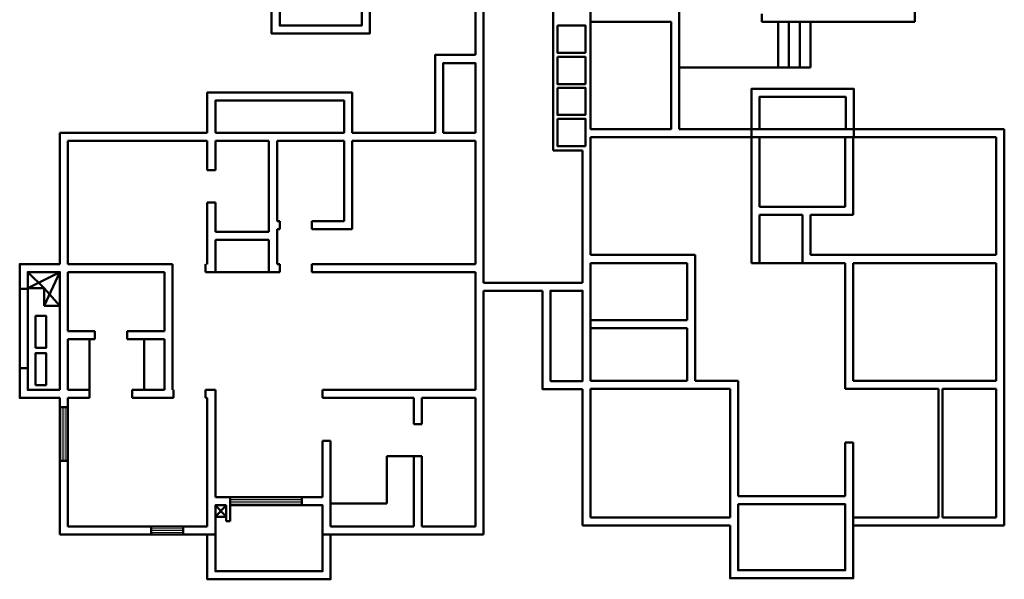
# Model space of a CAD drawing. Units: inches. Extents: x -105 to 1531, y -656 to 2003.
# Tile 1 of 6: x -105 to 997, y -656 to -29. Entities that reach past the tile are written whole.
import ezdxf

# ---------------------------------------------------------------- set-up
doc = ezdxf.new("R2010")
doc.units = ezdxf.units.IN
doc.header["$MEASUREMENT"] = 0
doc.layers.add('A-GLAZ', color=4, linetype='Continuous', lineweight=18)
doc.layers.add('A-WALL', color=7, linetype='Continuous', lineweight=50)

msp = doc.modelspace()

# ---------------------------------------------------------------- linework, layer by layer
at = {"layer": 'A-GLAZ'}
for p, q in [((105, -303), (102.8, -303)), ((105, -303), (102.8, -303)), ((102.8, -312), (105, -312)), ((-57.5, -523.3), (-57.5, -463.3)), ((-55.5, -523.3), (-55.5, -463.3)), ((-53.5, -523.3), (-53.5, -463.3)), ((-51, -463.3), (-51, -523.3)), ((130.5, -566.5), (210.6, -566.5)), ((130.5, -568.5), (210.6, -568.5)), ((130.5, -570.5), (210.6, -570.5)), ((42.1, -599.5), (78.1, -599.5)), ((42.1, -601.5), (78.1, -601.5)), ((42.1, -603.5), (78.1, -603.5))]:
    msp.add_line(p, q, dxfattribs=at)
at = {"layer": 'A-WALL'}
for p, q in [((897, -31.9), (897, 112.1)), ((492, -31.9), (492, 67.1)), ((534, -31.9), (534, 49.1)), ((633, -31.9), (633, 35.6)), ((277.8, -36), (277.8, 0)), ((405, -69), (405, 0)), ((414, 0), (414, -78)), ((492, -31.9), (492, -175.9)), ((534, -31.9), (534, -151.9)), ((624, -31.9), (534, -31.9)), ((633, -31.9), (633, -151.9)), ((725.8, -22.9), (725.8, -31.9)), ((897, -31.9), (725.8, -31.9)), ((744, -82.9), (744, -31.9)), ((756, -82.9), (756, -31.9)), ((768, -82.9), (768, -31.9)), ((780, -82.9), (780, -31.9)), ((405, -78), (369, -78)), ((369, -78), (369, -156)), ((405, -156), (405, -78)), ((414, -78), (414, -156)), ((780, -82.9), (633, -82.9)), ((258, -156), (258, -120)), ((723, -151.9), (723, -115.9)), ((534, -151.9), (624, -151.9)), ((633, -151.9), (997, -151.9)), ((997, -151.9), (997, -595.9)), ((-60, -156), (-60, -303)), ((105, -156), (-60, -156)), ((-51, -165), (-51, -303)), ((105, -165), (-51, -165)), ((105, -165), (105, -198)), ((258, -156), (114, -156)), ((114, -165), (114, -198)), ((174, -165), (114, -165)), ((174, -165), (174, -267)), ((183, -165), (183, -255)), ((258, -165), (183, -165)), ((258, -165), (258, -255)), ((360, -156), (267, -156)), ((405, -165), (267, -165)), ((267, -165), (267, -264)), ((405, -156), (369, -156)), ((405, -165), (405, -303)), ((414, -156), (414, -323.9)), ((534, -160.9), (534, -175.9)), ((633, -160.9), (534, -160.9)), ((534, -160.9), (714, -160.9)), ((534, -160.9), (534, -292.9)), ((714, -160.9), (714, -301.9)), ((723, -160.9), (723, -238.9)), ((723, -160.9), (819, -160.9)), ((819, -160.9), (819, -238.9)), ((828, -160.9), (828, -247.9)), ((828, -160.9), (988, -160.9)), ((988, -160.9), (988, -292.9)), ((492, -175.9), (525, -175.9)), ((525, -175.9), (525, -323.9)), ((534, -175.9), (534, -292.9)), ((114, -198), (105, -198)), ((105, -234), (114, -234)), ((105, -234), (105, -303)), ((114, -234), (114, -267)), ((723, -238.9), (819, -238.9)), ((723, -247.9), (771, -247.9)), ((723, -247.9), (723, -301.9)), ((771, -247.9), (771, -301.9)), ((780, -247.9), (780, -292.9)), ((780, -247.9), (828, -247.9)), ((186, -255), (183, -255)), ((183, -264), (183, -303)), ((186, -264), (183, -264)), ((186, -255), (186, -264)), ((258, -255), (222, -255)), ((222, -264), (222, -255)), ((267, -264), (222, -264)), ((174, -267), (114, -267)), ((174, -276), (114, -276)), ((114, -276), (114, -312)), ((174, -276), (174, -312)), ((534, -292.9), (651, -292.9)), ((651, -292.9), (651, -433.9)), ((780, -292.9), (988, -292.9)), ((66, -303), (-51, -303)), ((66, -312), (66, -303)), ((102.8, -303), (102.8, -312)), ((186, -303), (183, -303)), ((186, -303), (186, -312)), ((405, -303), (222, -303)), ((222, -312), (222, -303)), ((534, -301.9), (642, -301.9)), ((534, -301.9), (534, -365.9)), ((534, -301.9), (534, -332.9)), ((642, -301.9), (642, -365.9)), ((714, -301.9), (819, -301.9)), ((819, -301.9), (819, -442.9)), ((828, -301.9), (828, -433.9)), ((828, -301.9), (988, -301.9)), ((988, -301.9), (988, -433.9)), ((-60, -312), (-96, -312)), ((-96, -312), (-96, -330)), ((-60, -312), (-96, -330)), ((-96, -330), (-96, -312)), ((-96, -312), (-77.7, -330)), ((-77.7, -350), (-60, -312)), ((-60, -312), (-60, -444)), ((57, -312), (-51, -312)), ((-51, -312), (-51, -378)), ((57, -312), (57, -378)), ((66, -312), (66, -444)), ((186, -312), (102.8, -312)), ((405, -312), (222, -312)), ((405, -312), (405, -444)), ((-96, -330), (-77.7, -330)), ((-77.7, -330), (-77.7, -350)), ((-77.7, -330), (-60, -350)), ((525, -323.9), (414, -323.9)), ((-105, -330.8), (-96, -330.8)), ((-96, -330.8), (-96, -419.5)), ((480, -332.9), (414, -332.9)), ((414, -332.9), (414, -606)), ((525, -332.9), (489, -332.9)), ((525, -332.9), (525, -434.1)), ((534, -332.9), (534, -365.9)), ((-77.7, -350), (-60, -350)), ((-60, -350), (-77.7, -350)), ((534, -365.9), (642, -365.9)), ((-20.8, -378), (-51, -378)), ((-20.8, -387), (-20.8, -378)), ((57, -378), (15.2, -378)), ((15.2, -378), (15.2, -387)), ((534, -374.9), (642, -374.9)), ((534, -374.9), (534, -433.9)), ((534, -374.9), (534, -433.9)), ((642, -374.9), (642, -433.9)), ((-51, -387), (-51, -444)), ((-20.8, -387), (-51, -387)), ((-27, -444), (-27, -387)), ((57, -387), (15.2, -387)), ((34.2, -444), (34.2, -387)), ((57, -387), (57, -444)), ((-96, -419.5), (-105, -419.5)), ((525, -434.1), (489, -434.1)), ((534, -433.9), (642, -433.9)), ((651, -433.9), (699, -433.9)), ((699, -433.9), (699, -562.9)), ((828, -433.9), (988, -433.9)), ((-27, -444), (-51, -444)), ((-27, -453), (-27, -444)), ((57, -444), (21, -444)), ((21, -444), (21, -453)), ((67, -444), (66, -444)), ((67, -444), (67, -453)), ((114, -444), (103, -444)), ((103, -453), (103, -444)), ((114, -453), (114, -444)), ((405, -444), (234, -444)), ((234, -453), (234, -444)), ((234, -444), (234, -453)), ((525, -443.1), (525, -595.9)), ((534, -442.9), (690, -442.9)), ((534, -442.9), (534, -586.9)), ((534, -442.9), (534, -586.9)), ((690, -442.9), (690, -586.9)), ((828, -442.9), (819, -442.9)), ((828, -442.9), (923.5, -442.9)), ((923.5, -442.9), (923.5, -586.9)), ((928, -442.9), (928, -586.9)), ((928, -442.9), (988, -442.9)), ((988, -442.9), (988, -586.9)), ((-60, -453), (-60, -606)), ((-51, -453), (-51, -597)), ((-27, -453), (-51, -453)), ((67, -453), (21, -453)), ((105, -453), (103, -453)), ((105, -453), (103, -453)), ((105, -453), (105, -597)), ((114, -453), (114, -564)), ((234, -453), (243, -453)), ((336, -453), (243, -453)), ((336, -453), (336, -482.2)), ((405, -453), (345, -453)), ((345, -453), (345, -482.2)), ((405, -453), (405, -597)), ((-60, -463.3), (-51, -463.3)), ((336, -482.2), (345, -482.2)), ((234, -501), (234, -564)), ((243, -501), (234, -501)), ((243, -501), (243, -597)), ((243, -501), (243, -502)), ((243, -502), (243, -503)), ((819, -502.9), (828, -502.9)), ((819, -502.9), (819, -562.9)), ((828, -502.9), (828, -586.9)), ((-51, -523.3), (-60, -523.3)), ((336, -518.2), (306, -518.2)), ((306, -518.2), (306, -571.1)), ((345, -518.2), (336, -518.2)), ((336, -518.2), (336, -597)), ((345, -518.2), (345, -597)), ((234, -564), (114, -564)), ((114, -573), (114, -606)), ((114, -573), (114, -647)), ((114, -573), (126, -573)), ((126, -573), (114, -573)), ((114, -586), (126, -573)), ((126, -586), (114, -573)), ((126, -573), (126, -591)), ((126, -573), (126, -586)), ((130.5, -591), (130.5, -564)), ((130.5, -564), (130.5, -568.5)), ((234, -573), (130.5, -573)), ((210.6, -568.5), (210.6, -564)), ((210.6, -564), (210.6, -573)), ((234, -573), (234, -606)), ((306, -571.1), (243, -571.1)), ((699, -562.9), (819, -562.9)), ((699, -571.9), (819, -571.9)), ((699, -571.9), (699, -595.9)), ((819, -571.9), (819, -595.9)), ((819, -571.9), (819, -645.9)), ((126, -586), (114, -586)), ((126, -591), (130.5, -591)), ((534, -586.9), (690, -586.9)), ((828, -586.9), (923.5, -586.9)), ((928, -586.9), (988, -586.9)), ((105, -606), (-60, -606)), ((105, -597), (-51, -597)), ((42.1, -606), (42.1, -597)), ((54.1, -606), (42.1, -606)), ((78.1, -606), (54.1, -606)), ((78.1, -597), (78.1, -606)), ((105, -606), (114, -606)), ((243, -606), (234, -606)), ((336, -597), (243, -597)), ((414, -606), (243, -606)), ((405, -597), (345, -597)), ((525, -595.9), (690, -595.9)), ((828, -595.9), (997, -595.9))]:
    msp.add_line(p, q, dxfattribs=at)
for points in [[(286.8, 0), (286.8, -45), (177, -45), (177, 0)], [(360, -156), (360, -69), (405, -69)], [(414, -69), (414, -165)], [(267, -156), (267, -111), (105, -111), (105, -156)], [(114, -165), (174, -165)], [(183, -165), (258, -165)], [(405, -165), (360, -165)], [(-60, -453), (-105, -453), (-105, -303), (-60, -303)], [(-51, -312), (-51, -378)], [(525, -323.9), (480, -323.9)], [(534, -433.9), (534, -323.9)], [(480, -332.9), (480, -443.1), (525, -443.1)], [(-51, -387), (-51, -444)], [(534, -443.1), (534, -442.9)], [(105, -564), (105, -597)], [(234, -564), (114, -564)], [(126, -573), (114, -573), (114, -647), (234, -647), (234, -573), (130.5, -573)], [(243, -597), (243, -564)], [(690, -586.9), (690, -562.9)], [(828, -562.9), (828, -654.9), (690, -654.9), (690, -595.9)], [(699, -562.9), (819, -562.9)], [(105, -606), (105, -656), (243, -656), (243, -606)]]:
    msp.add_lwpolyline(points, dxfattribs=at)
for points in [[(186, 0), (277.8, 0), (277.8, -36), (186, -36)], [(534, -31.9), (624, -31.9), (624, -151.9), (534, -151.9)], [(496.9, -35.9), (528.2, -35.9), (528.2, -66.4), (496.9, -66.4)], [(496.9, -71.1), (528.2, -71.1), (528.2, -101.6), (496.9, -101.6)], [(405, -156), (369, -156), (369, -78), (405, -78)], [(496.9, -105.6), (528.2, -105.6), (528.2, -136.1), (496.9, -136.1)], [(828.6, -160.9), (714, -160.9), (714, -106.9), (828.6, -106.9)], [(114, -156), (258, -156), (258, -120), (114, -120)], [(819.6, -151.9), (723, -151.9), (723, -115.9), (819.6, -115.9)], [(496.9, -140.4), (528.2, -140.4), (528.2, -170.9), (496.9, -170.9)], [(-60, -444), (-96, -444), (-96, -312), (-60, -312)], [(489, -434.1), (525, -434.1), (525, -332.9), (489, -332.9)], [(-87.3, -396.9), (-75.4, -396.9), (-75.4, -361.1), (-87.3, -361.1)], [(-87.3, -438.5), (-75.4, -438.5), (-75.4, -402.7), (-87.3, -402.7)], [(699, -571.9), (819, -571.9), (819, -645.9), (699, -645.9)]]:
    msp.add_lwpolyline(points, close=True, dxfattribs=at)

doc.saveas('drawing.dxf')
